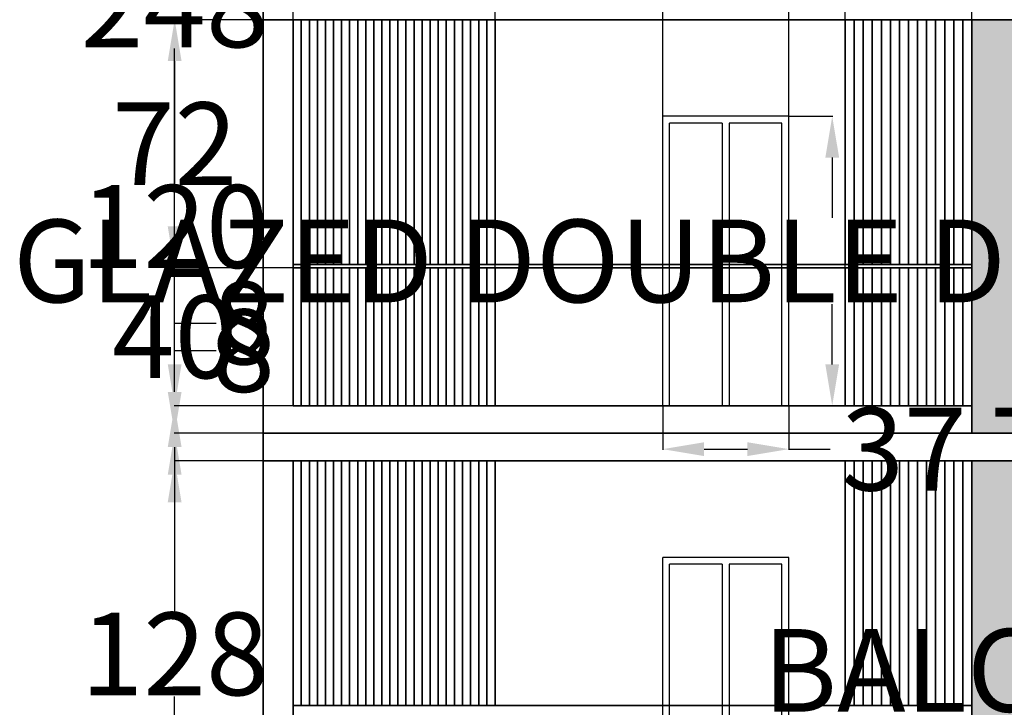
# Model space of a CAD drawing. Units: inches. Extents: x 172 to 828, y 190 to 777.
# Tile 2 of 9: x 188 to 474, y 408 to 607. Entities that reach past the tile are written whole.
import ezdxf

# ---------------------------------------------------------------- set-up
doc = ezdxf.new("R2010")
doc.units = ezdxf.units.IN
doc.header["$MEASUREMENT"] = 0
for name, color, linetype, lineweight in [('A-ANNO-DIMS', 2, 'Continuous', 18), ('A-DOOR', 4, 'Continuous', 25), ('A-ELEV', 7, 'Continuous', 35), ('A-ELEV-PATT', 8, 'Continuous', 13)]:
    doc.layers.add(name, color=color, linetype=linetype, lineweight=lineweight)
doc.styles.get("Standard").update_dxf_attribs({"font": 'arial.ttf'})
doc.dimstyles.get("Standard").update_dxf_attribs({"dimtxt": 24, "dimasz": 12, "dimexe": 0.18, "dimexo": 0.0625, "dimgap": 0.09, "dimtad": 0, "dimtih": 1, "dimtoh": 1, "dimdec": 0, "dimzin": 0, "dimdsep": 46, "dimlunit": 3, "dimtxsty": 'Standard', "dimcen": 0.09, "dimadec": 0, "dimazin": 0, "dimtfac": 1, "dimtdec": 0, "dimtofl": 0, "dimtmove": 0, "dimatfit": 3, "dimfxl": 1, "dimtolj": 1, "dimtzin": 0, "dimarcsym": 0})
pattern_1 = [(228.012788, (0.72, 1), (-8, -9), [0.134536, -13.319088]), (184.969741, (0.63, 0.9), (12, 1), [0.230868, -22.8559248]), (132.510447, (0.4, 0.88), (10, -11), [0.162788, -16.1160326]), (267.273689, (0.01, 0.63), (1, 20), [0.210238, -20.813558]), (292.833654, (0, 0.42), (-5, 12), [0.206155, -20.4093731]), (357.273689, (0.08, 0.23), (-20, 1), [0.210238, -20.813558]), (37.6942405, (0.29, 0.22), (-13, -10), [0.278029, -27.5248485]), (72.2553284, (0.51, 0.39), (7, 22), [0.262488, -25.9863215]), (121.4295656, (0.59, 0.64), (-8, 13), [0.21095, -20.8840731]), (175.236358, (0.48, 0.82), (11, -1), [0.240832, -11.8007626]), (222.397438, (0.24, 0.84), (-12, -11), [0.311448, -30.833375]), (138.814075, (1, 0.62), (-7, 6), [0.106301, -10.5238448]), (171.4692344, (0.92, 0.69), (13, -2), [0.202237, -20.0215114]), (225, (0.72, 0.72), (-1e-16, -1), [0.141421, -1.2727926]), (203.19859, (0.65, 0.84), (5, 2), [0.076158, -7.5396151]), (291.80141, (0.58, 0.81), (-1, 3), [0.107703, -5.2774618]), (30.963757, (0.62, 0.71), (3, 2), [0.174929, -5.6560229]), (161.56505, (0.77, 0.8), (2, -1), [0.126491, -3.0357867]), (16.38954, (0, 0.81), (10, 3), [0.1772, -17.5428451]), (70.346176, (0.17, 0.86), (-4, -11), [0.148661, -14.7174077]), (293.19859, (0.77, 1), (-2, 5), [0.152315, -7.4634581]), (343.61046, (0.83, 0.86), (-10, 3), [0.1772, -17.5428451]), (339.443955, (0, 0.19), (-5, 2), [0.17088, -8.3731237]), (294.775141, (0.16, 0.13), (-5, 11), [0.143178, -14.1746431]), (66.80141, (0.78, 0), (2, 5), [0.152315, -7.4634581]), (17.354025, (0.84, 0.14), (-13, -4), [0.167631, -16.5954236]), (69.443955, (0.29, 0), (-2, -5), [0.08544, -8.4585637]), (101.309932, (0.72, 0), (-1, 4), [0.05099, -5.0480295]), (165.963757, (0.71, 0.05), (3, -1), [0.206155, -3.9169506]), (186.009006, (0.51, 0.1), (10, 1), [0.19105, -18.9139232]), (303.690068, (0.62, 0.62), (-1, 2), [0.144222, -3.4613293]), (353.1572266, (0.7, 0.5), (17, -2), [0.251794, -24.9275626]), (60.945396, (0.95, 0.47), (-4, -7), [0.102956, -10.1926741]), (90, (1, 0.56), (-1, 1), [0.06, -0.94]), (120.256437, (0.49, 0.13), (4, -7), [0.138924, -13.75352]), (48.012788, (0.42, 0.25), (8, 9), [0.269072, -13.184552]), (0, (0.6, 0.45), (1, 1), [0.26, -0.74]), (325.3048465, (0.86, 0.45), (10, -7), [0.158114, -15.6532743]), (254.054604, (0.99, 0.36), (-1, -4), [0.145602, -7.1345079]), (207.6459754, (0.95, 0.22), (-19, -10), [0.237065, -23.4694742]), (175.426079, (0.74, 0.11), (-13, 1), [0.250799, -24.8290734])]

# ---------------------------------------------------------------- blocks, each defined once
blk = doc.blocks.new('DOOR-GLAZED-DBL')
for p, q in [((36.57, 84), (0, 84)), ((0, 0), (0, 84)), ((36.57, 0), (36.57, 84)), ((2, 0), (2, 82)), ((17.29, 82), (2, 82)), ((17.29, 82), (17.29, 0)), ((34.57, 82), (19.29, 82)), ((19.29, 82), (19.29, 0)), ((34.57, 0), (34.57, 82))]:
    blk.add_line(p, q)
blk = doc.blocks.new('*D4')
at = {"layer": 'A-ANNO-DIMS', "color": 0, "lineweight": -2, "transparency": 16777216}
for p, q in [((601.02, 471.8), (617.1, 471.8)), ((616.92, 459.8), (616.92, 431.1)), ((616.92, 377.39), (616.92, 406.09)), ((601.02, 365.39), (617.1, 365.39))]:
    blk.add_line(p, q, dxfattribs=at)
at = {"layer": 'A-ANNO-DIMS', "color": 0, "transparency": 16777216}
for points in [[(614.92, 459.8), (618.92, 459.8), (616.92, 471.8)], [(614.92, 377.39), (618.92, 377.39), (616.92, 365.39)]]:
    blk.add_solid(points, dxfattribs=at)
at = {"layer": 'Defpoints', "color": 0, "transparency": 16777216}
for p in [(600.96, 471.8), (616.92, 471.8), (600.96, 365.39)]:
    blk.add_point(p, dxfattribs=at)
at = {"layer": 'A-ANNO-DIMS', "color": 0, "transparency": 16777216, "insert": (616.92, 418.6), "char_height": 24, "attachment_point": 5}
blk.add_mtext('\\A1;BALCONY WINDOW 106 TYP.', dxfattribs=at)
blk = doc.blocks.new('*D6')
at = {"layer": 'A-ANNO-DIMS', "color": 0, "lineweight": -2, "transparency": 16777216}
for p, q in [((411.3, 579.39), (424.02, 579.39)), ((423.84, 567.39), (423.84, 549.9)), ((423.84, 507.39), (423.84, 524.88)), ((411.3, 495.39), (424.02, 495.39))]:
    blk.add_line(p, q, dxfattribs=at)
at = {"layer": 'A-ANNO-DIMS', "color": 0, "transparency": 16777216}
for points in [[(421.84, 567.39), (425.84, 567.39), (423.84, 579.39)], [(421.84, 507.39), (425.84, 507.39), (423.84, 495.39)]]:
    blk.add_solid(points, dxfattribs=at)
at = {"layer": 'Defpoints', "color": 0, "transparency": 16777216}
for p in [(411.24, 579.39), (423.84, 579.39), (411.24, 495.39)]:
    blk.add_point(p, dxfattribs=at)
at = {"layer": 'A-ANNO-DIMS', "color": 0, "transparency": 16777216, "insert": (423.84, 537.39), "char_height": 24, "attachment_point": 5}
blk.add_mtext('\\A1;GLAZED DOUBLE DOOR 84 TYP.', dxfattribs=at)
blk = doc.blocks.new('*D7')
at = {"layer": 'A-ANNO-DIMS', "color": 0, "lineweight": -2, "transparency": 16777216}
for p, q in [((374.66, 495.33), (374.66, 482.61)), ((411.24, 495.33), (411.24, 482.61)), ((386.66, 482.79), (399.24, 482.79)), ((411.24, 482.79), (423.24, 482.79))]:
    blk.add_line(p, q, dxfattribs=at)
at = {"layer": 'A-ANNO-DIMS', "color": 0, "transparency": 16777216}
for points in [[(386.66, 484.79), (386.66, 480.79), (374.66, 482.79)], [(399.24, 484.79), (399.24, 480.79), (411.24, 482.79)]]:
    blk.add_solid(points, dxfattribs=at)
at = {"layer": 'Defpoints', "color": 0, "transparency": 16777216}
for p in [(374.66, 495.39), (411.24, 495.39), (411.24, 482.79)]:
    blk.add_point(p, dxfattribs=at)
at = {"layer": 'A-ANNO-DIMS', "color": 0, "transparency": 16777216, "insert": (481.73, 482.79), "char_height": 24, "attachment_point": 5}
blk.add_mtext('\\A1;37 TYP.', dxfattribs=at)
blk = doc.blocks.new('*D10')
at = {"layer": 'A-ANNO-DIMS', "color": 0, "lineweight": -2, "transparency": 16777216}
for p, q in [((258.78, 231.45), (258.78, 761.27)), ((270.78, 761.09), (412.23, 761.09)), ((606.78, 761.09), (465.33, 761.09)), ((618.78, 735.45), (618.78, 761.27))]:
    blk.add_line(p, q, dxfattribs=at)
at = {"layer": 'A-ANNO-DIMS', "color": 0, "transparency": 16777216}
for points in [[(270.78, 763.09), (270.78, 759.09), (258.78, 761.09)], [(606.78, 763.09), (606.78, 759.09), (618.78, 761.09)]]:
    blk.add_solid(points, dxfattribs=at)
at = {"layer": 'Defpoints', "color": 0, "transparency": 16777216}
for p in [(618.78, 761.09), (618.78, 735.39), (258.78, 231.39)]:
    blk.add_point(p, dxfattribs=at)
at = {"layer": 'A-ANNO-DIMS', "color": 0, "transparency": 16777216, "insert": (438.78, 761.09), "char_height": 24, "attachment_point": 5}
blk.add_mtext('\\A1;360', dxfattribs=at)
blk = doc.blocks.new('*D13')
at = {"layer": 'A-ANNO-DIMS', "color": 0, "lineweight": -2, "transparency": 16777216}
for p, q in [((258.72, 487.39), (232.9, 487.39)), ((233.08, 475.39), (233.08, 435.74)), ((233.08, 371.39), (233.08, 411.05)), ((258.72, 359.39), (232.9, 359.39))]:
    blk.add_line(p, q, dxfattribs=at)
at = {"layer": 'A-ANNO-DIMS', "color": 0, "transparency": 16777216}
for points in [[(231.08, 475.39), (235.08, 475.39), (233.08, 487.39)], [(231.08, 371.39), (235.08, 371.39), (233.08, 359.39)]]:
    blk.add_solid(points, dxfattribs=at)
at = {"layer": 'Defpoints', "color": 0, "transparency": 16777216}
for p in [(233.08, 487.39), (258.78, 487.39), (258.78, 359.39)]:
    blk.add_point(p, dxfattribs=at)
at = {"layer": 'A-ANNO-DIMS', "color": 0, "transparency": 16777216, "insert": (233.08, 423.39), "char_height": 24, "attachment_point": 5}
blk.add_mtext('\\A1;128', dxfattribs=at)
blk = doc.blocks.new('*D14')
at = {"layer": 'A-ANNO-DIMS', "color": 0, "lineweight": -2, "transparency": 16777216}
for p, q in [((258.72, 735.39), (232.9, 735.39)), ((233.08, 723.39), (233.08, 623.74)), ((233.08, 499.39), (233.08, 599.05)), ((258.72, 487.39), (232.9, 487.39))]:
    blk.add_line(p, q, dxfattribs=at)
at = {"layer": 'A-ANNO-DIMS', "color": 0, "transparency": 16777216}
for points in [[(231.08, 723.39), (235.08, 723.39), (233.08, 735.39)], [(231.08, 499.39), (235.08, 499.39), (233.08, 487.39)]]:
    blk.add_solid(points, dxfattribs=at)
at = {"layer": 'Defpoints', "color": 0, "transparency": 16777216}
for p in [(233.08, 735.39), (258.78, 735.39), (258.78, 487.39)]:
    blk.add_point(p, dxfattribs=at)
at = {"layer": 'A-ANNO-DIMS', "color": 0, "transparency": 16777216, "insert": (233.08, 611.39), "char_height": 24, "attachment_point": 5}
blk.add_mtext('\\A1;248', dxfattribs=at)
blk = doc.blocks.new('*D67')
at = {"layer": 'A-ANNO-DIMS', "color": 0, "lineweight": -2, "transparency": 16777216}
for p, q in [((233.08, 499.39), (233.08, 511.39)), ((233.08, 511.39), (245.08, 511.39)), ((258.72, 487.39), (232.9, 487.39)), ((258.72, 479.39), (232.9, 479.39)), ((233.08, 467.39), (233.08, 455.39))]:
    blk.add_line(p, q, dxfattribs=at)
at = {"layer": 'A-ANNO-DIMS', "color": 0, "transparency": 16777216}
for points in [[(231.08, 499.39), (235.08, 499.39), (233.08, 487.39)], [(231.08, 467.39), (235.08, 467.39), (233.08, 479.39)]]:
    blk.add_solid(points, dxfattribs=at)
at = {"layer": 'Defpoints', "color": 0, "transparency": 16777216}
for p in [(233.08, 487.39), (258.78, 487.39), (258.78, 479.39)]:
    blk.add_point(p, dxfattribs=at)
at = {"layer": 'A-ANNO-DIMS', "color": 0, "transparency": 16777216, "insert": (253.08, 511.39), "char_height": 24, "attachment_point": 5}
blk.add_mtext('\\A1;8', dxfattribs=at)
blk = doc.blocks.new('*D68')
at = {"layer": 'A-ANNO-DIMS', "color": 0, "lineweight": -2, "transparency": 16777216}
for p, q in [((258.72, 607.39), (232.9, 607.39)), ((233.08, 595.39), (233.08, 559.74)), ((233.08, 499.39), (233.08, 535.05)), ((258.72, 487.39), (232.9, 487.39))]:
    blk.add_line(p, q, dxfattribs=at)
at = {"layer": 'A-ANNO-DIMS', "color": 0, "transparency": 16777216}
for points in [[(231.08, 595.39), (235.08, 595.39), (233.08, 607.39)], [(231.08, 499.39), (235.08, 499.39), (233.08, 487.39)]]:
    blk.add_solid(points, dxfattribs=at)
at = {"layer": 'Defpoints', "color": 0, "transparency": 16777216}
for p in [(233.08, 607.39), (258.78, 607.39), (258.78, 487.39)]:
    blk.add_point(p, dxfattribs=at)
at = {"layer": 'A-ANNO-DIMS', "color": 0, "transparency": 16777216, "insert": (233.08, 547.39), "char_height": 24, "attachment_point": 5}
blk.add_mtext('\\A1;120', dxfattribs=at)
blk = doc.blocks.new('*D69')
at = {"layer": 'A-ANNO-DIMS', "color": 0, "lineweight": -2, "transparency": 16777216}
for p, q in [((233.08, 627.39), (233.08, 639.39)), ((233.08, 639.39), (245.08, 639.39)), ((267.42, 615.39), (232.9, 615.39)), ((258.72, 607.39), (232.9, 607.39)), ((233.08, 595.39), (233.08, 583.39))]:
    blk.add_line(p, q, dxfattribs=at)
at = {"layer": 'A-ANNO-DIMS', "color": 0, "transparency": 16777216}
for points in [[(231.08, 627.39), (235.08, 627.39), (233.08, 615.39)], [(231.08, 595.39), (235.08, 595.39), (233.08, 607.39)]]:
    blk.add_solid(points, dxfattribs=at)
at = {"layer": 'Defpoints', "color": 0, "transparency": 16777216}
for p in [(233.08, 615.39), (267.48, 615.39), (258.78, 607.39)]:
    blk.add_point(p, dxfattribs=at)
at = {"layer": 'A-ANNO-DIMS', "color": 0, "transparency": 16777216, "insert": (253.08, 639.39), "char_height": 24, "attachment_point": 5}
blk.add_mtext('\\A1;8', dxfattribs=at)
blk = doc.blocks.new('*D70')
at = {"layer": 'A-ANNO-DIMS', "color": 0, "lineweight": -2, "transparency": 16777216}
for p, q in [((233.08, 507.39), (233.08, 519.39)), ((233.08, 519.39), (245.08, 519.39)), ((267.42, 495.39), (232.9, 495.39)), ((258.72, 487.39), (232.9, 487.39)), ((233.08, 475.39), (233.08, 463.39))]:
    blk.add_line(p, q, dxfattribs=at)
at = {"layer": 'A-ANNO-DIMS', "color": 0, "transparency": 16777216}
for points in [[(231.08, 507.39), (235.08, 507.39), (233.08, 495.39)], [(231.08, 475.39), (235.08, 475.39), (233.08, 487.39)]]:
    blk.add_solid(points, dxfattribs=at)
at = {"layer": 'Defpoints', "color": 0, "transparency": 16777216}
for p in [(233.08, 495.39), (267.48, 495.39), (258.78, 487.39)]:
    blk.add_point(p, dxfattribs=at)
at = {"layer": 'A-ANNO-DIMS', "color": 0, "transparency": 16777216, "insert": (253.08, 519.39), "char_height": 24, "attachment_point": 5}
blk.add_mtext('\\A1;8', dxfattribs=at)
blk = doc.blocks.new('*D71')
at = {"layer": 'A-ANNO-DIMS', "color": 0, "lineweight": -2, "transparency": 16777216}
for p, q in [((233.079175, 547.392291), (233.079175, 559.392291)), ((267.419715, 535.392291), (232.899175, 535.392291)), ((267.419715, 495.392291), (232.899175, 495.392291)), ((233.079175, 483.392291), (233.079175, 471.392291))]:
    blk.add_line(p, q, dxfattribs=at)
at = {"layer": 'A-ANNO-DIMS', "color": 0, "transparency": 16777216}
for points in [[(231.079175, 547.392291), (235.079175, 547.392291), (233.079175, 535.392291)], [(231.079175, 483.392291), (235.079175, 483.392291), (233.079175, 495.392291)]]:
    blk.add_solid(points, dxfattribs=at)
at = {"layer": 'Defpoints', "color": 0, "transparency": 16777216}
for p in [(233.079175, 535.392291), (267.482215, 535.392291), (267.482215, 495.392291)]:
    blk.add_point(p, dxfattribs=at)
at = {"layer": 'A-ANNO-DIMS', "color": 0, "transparency": 16777216, "insert": (233.079175, 515.392291), "char_height": 24, "attachment_point": 5}
blk.add_mtext('\\A1;40', dxfattribs=at)
blk = doc.blocks.new('*D72')
at = {"layer": 'A-ANNO-DIMS', "color": 0, "lineweight": -2, "transparency": 16777216}
for p, q in [((267.42, 607.39), (232.9, 607.39)), ((233.08, 595.39), (233.08, 583.53)), ((233.08, 547.39), (233.08, 559.25)), ((267.42, 535.39), (232.9, 535.39))]:
    blk.add_line(p, q, dxfattribs=at)
at = {"layer": 'A-ANNO-DIMS', "color": 0, "transparency": 16777216}
for points in [[(231.08, 595.39), (235.08, 595.39), (233.08, 607.39)], [(231.08, 547.39), (235.08, 547.39), (233.08, 535.39)]]:
    blk.add_solid(points, dxfattribs=at)
at = {"layer": 'Defpoints', "color": 0, "transparency": 16777216}
for p in [(233.08, 607.39), (267.48, 607.39), (267.48, 535.39)]:
    blk.add_point(p, dxfattribs=at)
at = {"layer": 'A-ANNO-DIMS', "color": 0, "transparency": 16777216, "insert": (233.08, 571.39), "char_height": 24, "attachment_point": 5}
blk.add_mtext('\\A1;72', dxfattribs=at)
blk = doc.blocks.new('*D73')
at = {"layer": 'A-ANNO-DIMS', "color": 0, "lineweight": -2, "transparency": 16777216}
for p, q in [((246.78, 761.09), (234.78, 761.09)), ((258.78, 607.45), (258.78, 761.27)), ((267.48, 495.45), (267.48, 761.27)), ((279.48, 761.09), (291.48, 761.09))]:
    blk.add_line(p, q, dxfattribs=at)
at = {"layer": 'A-ANNO-DIMS', "color": 0, "transparency": 16777216}
for points in [[(246.78, 763.09), (246.78, 759.09), (258.78, 761.09)], [(279.48, 763.09), (279.48, 759.09), (267.48, 761.09)]]:
    blk.add_solid(points, dxfattribs=at)
at = {"layer": 'Defpoints', "color": 0, "transparency": 16777216}
for p in [(267.48, 761.09), (258.78, 607.39), (267.48, 495.39)]:
    blk.add_point(p, dxfattribs=at)
at = {"layer": 'A-ANNO-DIMS', "color": 0, "transparency": 16777216, "insert": (332.08, 761.09), "char_height": 24, "attachment_point": 5}
blk.add_mtext('\\A1;8.703', dxfattribs=at)
blk = doc.blocks.new('*D74')
at = {"layer": 'A-ANNO-DIMS', "color": 0, "lineweight": -2, "transparency": 16777216}
for p, q in [((267.48, 495.45), (267.48, 761.27)), ((279.48, 761.09), (314.08, 761.09)), ((326.08, 495.45), (326.08, 761.27)), ((326.08, 761.09), (338.08, 761.09))]:
    blk.add_line(p, q, dxfattribs=at)
at = {"layer": 'A-ANNO-DIMS', "color": 0, "transparency": 16777216}
for points in [[(279.48, 763.09), (279.48, 759.09), (267.48, 761.09)], [(314.08, 763.09), (314.08, 759.09), (326.08, 761.09)]]:
    blk.add_solid(points, dxfattribs=at)
at = {"layer": 'Defpoints', "color": 0, "transparency": 16777216}
for p in [(326.08, 761.09), (267.48, 495.39), (326.08, 495.39)]:
    blk.add_point(p, dxfattribs=at)
at = {"layer": 'A-ANNO-DIMS', "color": 0, "transparency": 16777216, "insert": (378.68, 761.09), "char_height": 24, "attachment_point": 5}
blk.add_mtext('\\A1;58.59', dxfattribs=at)
blk = doc.blocks.new('*D75')
at = {"layer": 'A-ANNO-DIMS', "color": 0, "lineweight": -2, "transparency": 16777216}
for p, q in [((326.08, 495.45), (326.08, 761.27)), ((338.08, 761.09), (362.66, 761.09)), ((374.66, 495.45), (374.66, 761.27)), ((374.66, 761.09), (386.66, 761.09))]:
    blk.add_line(p, q, dxfattribs=at)
at = {"layer": 'A-ANNO-DIMS', "color": 0, "transparency": 16777216}
for points in [[(338.08, 763.09), (338.08, 759.09), (326.08, 761.09)], [(362.66, 763.09), (362.66, 759.09), (374.66, 761.09)]]:
    blk.add_solid(points, dxfattribs=at)
at = {"layer": 'Defpoints', "color": 0, "transparency": 16777216}
for p in [(374.66, 761.09), (326.08, 495.39), (374.66, 495.39)]:
    blk.add_point(p, dxfattribs=at)
at = {"layer": 'A-ANNO-DIMS', "color": 0, "transparency": 16777216, "insert": (427.75, 761.09), "char_height": 24, "attachment_point": 5}
blk.add_mtext('\\A1;48.59', dxfattribs=at)
blk = doc.blocks.new('*D76')
at = {"layer": 'A-ANNO-DIMS', "color": 0, "lineweight": -2, "transparency": 16777216}
for p, q in [((399.24, 761.09), (387.24, 761.09)), ((411.24, 495.45), (411.24, 761.27)), ((427.59, 495.45), (427.59, 761.27)), ((439.59, 761.09), (451.59, 761.09))]:
    blk.add_line(p, q, dxfattribs=at)
at = {"layer": 'A-ANNO-DIMS', "color": 0, "transparency": 16777216}
for points in [[(399.24, 763.09), (399.24, 759.09), (411.24, 761.09)], [(439.59, 763.09), (439.59, 759.09), (427.59, 761.09)]]:
    blk.add_solid(points, dxfattribs=at)
at = {"layer": 'Defpoints', "color": 0, "transparency": 16777216}
for p in [(427.59, 761.09), (411.24, 495.39), (427.59, 495.39)]:
    blk.add_point(p, dxfattribs=at)
at = {"layer": 'A-ANNO-DIMS', "color": 0, "transparency": 16777216, "insert": (500.36, 761.09), "char_height": 24, "attachment_point": 5}
blk.add_mtext('\\A1;16.356', dxfattribs=at)
blk = doc.blocks.new('*D77')
at = {"layer": 'A-ANNO-DIMS', "color": 0, "lineweight": -2, "transparency": 16777216}
for p, q in [((427.59, 495.45), (427.59, 761.27)), ((439.59, 761.09), (452.34, 761.09)), ((464.34, 495.45), (464.34, 761.27)), ((464.34, 761.09), (476.34, 761.09))]:
    blk.add_line(p, q, dxfattribs=at)
at = {"layer": 'A-ANNO-DIMS', "color": 0, "transparency": 16777216}
for points in [[(439.59, 763.09), (439.59, 759.09), (427.59, 761.09)], [(452.34, 763.09), (452.34, 759.09), (464.34, 761.09)]]:
    blk.add_solid(points, dxfattribs=at)
at = {"layer": 'Defpoints', "color": 0, "transparency": 16777216}
for p in [(464.34, 761.09), (427.59, 495.39), (464.34, 495.39)]:
    blk.add_point(p, dxfattribs=at)
at = {"layer": 'A-ANNO-DIMS', "color": 0, "transparency": 16777216, "insert": (516.86, 761.09), "char_height": 24, "attachment_point": 5}
blk.add_mtext('\\A1;36.74', dxfattribs=at)

msp = doc.modelspace()

# ---------------------------------------------------------------- hatches: boundary and pattern name
at = {"layer": 'A-ELEV-PATT'}
h = msp.add_hatch(dxfattribs=at)
h.set_pattern_fill('GRAVEL', color=256)
h.set_pattern_definition(pattern_1)
h.paths.add_polyline_path([(438.7792, 351.3923), (414.7792, 351.3923), (414.7792, 249.3923), (438.7792, 249.3923)])
h.paths.add_polyline_path([(480.7792, 351.3923), (456.7792, 351.3923), (456.7792, 249.3923), (480.7792, 249.3923)])
h.paths.add_polyline_path([(488.4232, 479.3923), (472.3356, 479.3923), (472.3356, 359.3923), (488.4232, 359.3923)])
h.paths.add_polyline_path([(488.4232, 607.3923), (472.3356, 607.3923), (472.3356, 487.3923), (488.4232, 487.3923)])
h = msp.add_hatch(dxfattribs=at)
h.set_pattern_fill('GRAVEL', color=256)
h.set_pattern_definition(pattern_1)
h.paths.add_polyline_path([(480.7792, 351.3923), (456.7792, 351.3923), (456.7792, 249.3923), (480.7792, 249.3923)])
h.paths.add_polyline_path([(488.4232, 479.3923), (472.3356, 479.3923), (472.3356, 359.3923), (488.4232, 359.3923)])
h.paths.add_polyline_path([(488.4232, 607.3923), (472.3356, 607.3923), (472.3356, 487.3923), (488.4232, 487.3923)])
h = msp.add_hatch(dxfattribs=at)
h.set_pattern_fill('GRAVEL', color=256, scale=20)
h.set_pattern_definition([(228.01279, (14.4, 20), (-160, -180), [2.69072, -266.38176]), (184.96974, (12.6, 18), (240, 20), [4.61736, -457.1185]), (132.51045, (8, 17.6), (200, -220), [3.25576, -322.32065]), (267.27369, (0.2, 12.6), (20, 400), [4.20476, -416.27116]), (292.83365, (0, 8.4), (-100, 240), [4.1231, -408.18746]), (357.27369, (1.6, 4.6), (-400, 20), [4.20476, -416.27116]), (37.69424, (5.8, 4.4), (-260, -200), [5.56058, -550.49697]), (72.25533, (10.2, 7.8), (140, 440), [5.24976, -519.72643]), (121.42957, (11.8, 12.8), (-160, 260), [4.219, -417.68146]), (175.23636, (9.6, 16.4), (220, -20), [4.81664, -236.01525]), (222.39744, (4.8, 16.8), (-240, -220), [6.22896, -616.6675]), (138.81407, (20, 12.4), (-140, 120), [2.126, -210.4769]), (171.46923, (18.4, 13.8), (260, -40), [4.04474, -400.43023]), (225, (14.4, 14.4), (-2e-15, -20), [2.8284, -25.45585]), (203.1986, (13, 16.8), (100, 40), [1.52316, -150.7923]), (291.8014, (11.6, 16.2), (-20, 60), [2.15406, -105.54924]), (30.96376, (12.4, 14.2), (60, 40), [3.4986, -113.12046]), (161.56505, (15.4, 16), (40, -20), [2.5298, -60.71573]), (16.38954, (0, 16.2), (200, 60), [3.544, -350.8569]), (70.34618, (3.4, 17.2), (-80, -220), [2.97322, -294.34815]), (293.1986, (15.4, 20), (-40, 100), [3.0463, -149.26916]), (343.61046, (16.6, 17.2), (-200, 60), [3.544, -350.8569]), (339.44395, (0, 3.8), (-100, 40), [3.4176, -167.46247]), (294.77514, (3.2, 2.6), (-100, 220), [2.86356, -283.49286]), (66.8014, (15.6, 0), (40, 100), [3.0463, -149.26916]), (17.35402, (16.8, 2.8), (-260, -80), [3.35262, -331.90847]), (69.44395, (5.8, 0), (-40, -100), [1.7088, -169.17127]), (101.30993, (14.4, 0), (-20, 80), [1.0198, -100.9606]), (165.96376, (14.2, 1), (60, -20), [4.1231, -78.339]), (186.009, (10.2, 2), (200, 20), [3.821, -378.27846]), (303.6901, (12.4, 12.4), (-20, 40), [2.88444, -69.2266]), (353.15723, (14, 10), (340, -40), [5.03588, -498.55125]), (60.9454, (19, 9.4), (-80, -140), [2.0591, -203.8535]), (90, (20, 11.2), (-20, 20), [1.2, -18.8]), (120.25644, (9.8, 2.6), (80, -140), [2.77848, -275.0704]), (48.01279, (8.4, 5), (160, 180), [5.38144, -263.69104]), (0, (12, 9), (20, 20), [5.2, -14.8]), (325.30485, (17.2, 9), (200, -140), [3.16228, -313.0655]), (254.0546, (19.8, 7.2), (-20, -80), [2.91204, -142.69016]), (207.64598, (19, 4.4), (-380, -200), [4.7413, -469.38948]), (175.42608, (14.8, 2.2), (-260, 20), [5.01598, -496.58147])])
h.paths.add_polyline_path([(480.7792, 351.3923), (456.7792, 351.3923), (456.7792, 249.3923), (480.7792, 249.3923)])
h.paths.add_polyline_path([(472.3356, 479.3923), (464.3356, 479.3923), (464.3356, 359.3923), (472.3356, 359.3923)])
h.paths.add_polyline_path([(488.4232, 479.3923), (472.3356, 479.3923), (472.3356, 359.3923), (488.4232, 359.3923)])
h.paths.add_polyline_path([(472.3356, 607.3923), (464.3356, 607.3923), (464.3356, 487.3923), (472.3356, 487.3923)])
h.paths.add_polyline_path([(488.4232, 607.3923), (472.3356, 607.3923), (472.3356, 487.3923), (488.4232, 487.3923)])

# ---------------------------------------------------------------- linework, layer by layer
at = {"layer": 'A-ELEV'}
for p, q in [((258.7792, 487.3923), (258.7792, 735.3923)), ((606.8158, 607.3923), (258.7792, 607.3923)), ((606.8158, 607.3923), (258.7792, 607.3923)), ((267.4822, 495.3923), (267.4822, 607.3923)), ((269.8186, 536.3923), (269.8186, 607.3923)), ((272.155, 536.3923), (272.155, 607.3923)), ((274.4914, 536.3923), (274.4914, 607.3923)), ((276.8278, 536.3923), (276.8278, 607.3923)), ((279.1642, 536.3923), (279.1642, 607.3923)), ((281.5006, 536.3923), (281.5006, 607.3923)), ((283.837, 536.3923), (283.837, 607.3923)), ((286.1735, 536.3923), (286.1735, 607.3923)), ((288.5099, 536.3923), (288.5099, 607.3923)), ((290.8463, 536.3923), (290.8463, 607.3923)), ((293.1827, 536.3923), (293.1827, 607.3923)), ((295.5191, 536.3923), (295.5191, 607.3923)), ((297.8555, 536.3923), (297.8555, 607.3923)), ((300.1919, 536.3923), (300.1919, 607.3923)), ((302.5283, 536.3923), (302.5283, 607.3923)), ((304.8647, 536.3923), (304.8647, 607.3923)), ((307.2011, 536.3923), (307.2011, 607.3923)), ((309.5375, 536.3923), (309.5375, 607.3923)), ((311.8739, 536.3923), (311.8739, 607.3923)), ((314.2715, 536.3923), (314.2715, 607.3923)), ((316.6079, 536.3923), (316.6079, 607.3923)), ((318.9443, 536.3923), (318.9443, 607.3923)), ((321.3419, 536.3923), (321.3419, 607.3923)), ((323.6783, 536.3923), (323.6783, 607.3923)), ((326.0147, 536.3923), (326.0147, 607.3923)), ((427.5926, 607.3923), (427.5926, 536.3923)), ((427.5926, 536.3923), (427.5926, 607.3923)), ((430.2171, 607.3923), (430.2171, 536.3923)), ((432.8416, 607.3923), (432.8416, 536.3923)), ((435.4661, 607.3923), (435.4661, 536.3923)), ((438.0906, 607.3923), (438.0906, 536.3923)), ((440.7151, 607.3923), (440.7151, 536.3923)), ((443.3396, 607.3923), (443.3396, 536.3923)), ((445.9641, 607.3923), (445.9641, 536.3923)), ((448.5886, 607.3923), (448.5886, 536.3923)), ((451.2131, 607.3923), (451.2131, 536.3923)), ((453.8376, 607.3923), (453.8376, 536.3923)), ((456.4621, 607.3923), (456.4621, 536.3923)), ((459.0866, 607.3923), (459.0866, 536.3923)), ((461.7111, 607.3923), (461.7111, 536.3923)), ((464.3356, 607.3923), (464.3356, 487.3923)), ((464.3356, 536.3923), (267.4822, 536.3923)), ((464.3356, 535.3923), (267.4822, 535.3923)), ((269.8186, 495.3923), (269.8186, 535.3923)), ((272.155, 495.3923), (272.155, 535.3923)), ((274.4914, 495.3923), (274.4914, 535.3923)), ((276.8278, 495.3923), (276.8278, 535.3923)), ((279.1642, 495.3923), (279.1642, 535.3923)), ((281.5006, 495.3923), (281.5006, 535.3923)), ((283.837, 495.3923), (283.837, 535.3923)), ((286.1735, 495.3923), (286.1735, 535.3923)), ((288.5099, 495.3923), (288.5099, 535.3923)), ((290.8463, 495.3923), (290.8463, 535.3923)), ((293.1827, 495.3923), (293.1827, 535.3923)), ((295.5191, 495.3923), (295.5191, 535.3923)), ((297.8555, 495.3923), (297.8555, 535.3923)), ((300.1919, 495.3923), (300.1919, 535.3923)), ((302.5283, 495.3923), (302.5283, 535.3923)), ((304.8647, 495.3923), (304.8647, 535.3923)), ((307.2011, 495.3923), (307.2011, 535.3923)), ((309.5375, 495.3923), (309.5375, 535.3923)), ((311.8739, 495.3923), (311.8739, 535.3923)), ((314.2715, 495.3923), (314.2715, 535.3923)), ((316.6079, 495.3923), (316.6079, 535.3923)), ((318.9443, 495.3923), (318.9443, 535.3923)), ((321.3419, 495.3923), (321.3419, 535.3923)), ((323.6783, 495.3923), (323.6783, 535.3923)), ((326.0759, 495.3923), (326.0759, 535.3923)), ((427.5926, 495.3923), (427.5926, 535.3923)), ((427.5926, 535.3923), (427.5926, 495.3923)), ((430.2171, 535.3923), (430.2171, 495.3923)), ((432.8416, 535.3923), (432.8416, 495.3923)), ((435.4661, 535.3923), (435.4661, 495.3923)), ((438.0906, 535.3923), (438.0906, 495.3923)), ((440.7151, 535.3923), (440.7151, 495.3923)), ((443.3396, 535.3923), (443.3396, 495.3923)), ((445.9641, 535.3923), (445.9641, 495.3923)), ((448.5886, 535.3923), (448.5886, 495.3923)), ((451.2131, 535.3923), (451.2131, 495.3923)), ((453.8376, 535.3923), (453.8376, 495.3923)), ((456.4621, 535.3923), (456.4621, 495.3923)), ((459.0866, 535.3923), (459.0866, 495.3923)), ((461.7111, 535.3923), (461.7111, 495.3923)), ((464.3356, 495.3923), (267.4822, 495.3923)), ((606.8158, 487.3923), (258.7792, 487.3923)), ((258.7792, 487.3923), (258.7792, 359.3923)), ((472.3356, 487.3923), (393.1206, 487.3923)), ((606.8158, 479.3923), (258.7792, 479.3923)), ((258.7792, 359.3923), (258.7792, 479.3923)), ((267.4822, 367.3923), (267.4822, 479.3923)), ((269.8186, 408.3923), (269.8186, 479.3923)), ((272.155, 408.3923), (272.155, 479.3923)), ((274.4914, 408.3923), (274.4914, 479.3923)), ((276.8278, 408.3923), (276.8278, 479.3923)), ((279.1642, 408.3923), (279.1642, 479.3923)), ((281.5006, 408.3923), (281.5006, 479.3923)), ((283.837, 408.3923), (283.837, 479.3923)), ((286.1735, 408.3923), (286.1735, 479.3923)), ((288.5099, 408.3923), (288.5099, 479.3923)), ((290.8463, 408.3923), (290.8463, 479.3923)), ((293.1827, 408.3923), (293.1827, 479.3923)), ((295.5191, 408.3923), (295.5191, 479.3923)), ((297.8555, 408.3923), (297.8555, 479.3923)), ((300.1919, 408.3923), (300.1919, 479.3923)), ((302.5283, 408.3923), (302.5283, 479.3923)), ((304.8647, 408.3923), (304.8647, 479.3923)), ((307.2011, 408.3923), (307.2011, 479.3923)), ((309.5375, 408.3923), (309.5375, 479.3923)), ((311.8739, 408.3923), (311.8739, 479.3923)), ((314.2715, 408.3923), (314.2715, 479.3923)), ((316.6079, 408.3923), (316.6079, 479.3923)), ((318.9443, 408.3923), (318.9443, 479.3923)), ((321.3419, 408.3923), (321.3419, 479.3923)), ((323.6783, 408.3923), (323.6783, 479.3923)), ((326.0147, 408.3923), (326.0147, 479.3923)), ((427.5926, 479.3923), (427.5926, 408.3923)), ((427.5926, 408.3923), (427.5926, 479.3923)), ((430.2171, 479.3923), (430.2171, 408.3923)), ((432.8416, 479.3923), (432.8416, 408.3923)), ((435.4661, 479.3923), (435.4661, 408.3923)), ((438.0906, 479.3923), (438.0906, 408.3923)), ((440.7151, 479.3923), (440.7151, 408.3923)), ((443.3396, 479.3923), (443.3396, 408.3923)), ((445.9641, 479.3923), (445.9641, 408.3923)), ((448.5886, 479.3923), (448.5886, 408.3923)), ((451.2131, 479.3923), (451.2131, 408.3923)), ((453.8376, 479.3923), (453.8376, 408.3923)), ((456.4621, 479.3923), (456.4621, 408.3923)), ((459.0866, 479.3923), (459.0866, 408.3923)), ((461.7111, 479.3923), (461.7111, 408.3923)), ((464.3356, 479.3923), (464.3356, 359.3923)), ((464.3356, 408.3923), (267.4822, 408.3923))]:
    msp.add_line(p, q, dxfattribs=at)

# ---------------------------------------------------------------- block references
at = {"layer": 'A-DOOR'}
for p in [(374.663, 495.392), (374.663, 367.392)]:
    msp.add_blockref('DOOR-GLAZED-DBL', p, dxfattribs=at)

# ---------------------------------------------------------------- dimensions: what is measured, and where the dimension line sits
at = {"layer": 'A-ANNO-DIMS'}
for base, p1, p2, override, picture, middle in [((267.4822, 761.0923), (258.7792, 607.3923), (267.4822, 495.3923), {"dimdec": 3, "dimlfac": 1, "dimrnd": 0, "dimzin": 0, "dimdsep": 46, "dimlunit": 2}, '*D73', (332.0824, 761.0923)), ((618.7792, 761.0923), (258.7792, 231.3923), (618.7792, 735.3923), {"dimdec": 0, "dimlfac": 1, "dimrnd": 0, "dimzin": 0, "dimdsep": 46, "dimlunit": 2}, '*D10', (438.7792, 761.0923)), ((326.0759, 761.0923), (267.4822, 495.3923), (326.0759, 495.3923), {"dimdec": 2, "dimlfac": 1, "dimrnd": 0, "dimzin": 0, "dimdsep": 46, "dimlunit": 2}, '*D74', (378.6843, 761.0923)), ((374.6632, 761.0923), (326.0759, 495.3923), (374.6632, 495.3923), {"dimdec": 2, "dimlfac": 1, "dimrnd": 0, "dimzin": 0, "dimdsep": 46, "dimlunit": 2}, '*D75', (427.7546, 761.0923)), ((427.5926, 761.0923), (411.2362, 495.3923), (427.5926, 495.3923), {"dimdec": 3, "dimlfac": 1, "dimrnd": 0, "dimzin": 0, "dimdsep": 46, "dimlunit": 2}, '*D76', (500.362, 761.0923)), ((464.3356, 761.0923), (427.5926, 495.3923), (464.3356, 495.3923), {"dimdec": 2, "dimlfac": 1, "dimrnd": 0, "dimzin": 0, "dimdsep": 46, "dimlunit": 2}, '*D77', (516.8622, 761.0923))]:
    dim = msp.add_linear_dim(base=base, p1=p1, p2=p2, dimstyle='Standard', override=override, dxfattribs=at)
    dim.commit()
    dim.dimension.update_dxf_attribs({"geometry": picture, "text_midpoint": middle})
for base, p1, p2, picture, middle in [((233.0792, 735.3923), (258.7792, 487.3923), (258.7792, 735.3923), '*D14', (233.0792, 611.3923)), ((233.0792, 615.3923), (258.7792, 607.3923), (267.4822, 615.3923), '*D69', (253.0764, 639.3923)), ((233.0792, 607.3923), (258.7792, 487.3923), (258.7792, 607.3923), '*D68', (233.0792, 547.3923)), ((233.0792, 607.3923), (267.4822, 535.3923), (267.4822, 607.3923), '*D72', (233.0792, 571.3923)), ((233.0792, 535.3923), (267.4822, 495.3923), (267.4822, 535.3923), '*D71', (233.0792, 515.3923)), ((233.0792, 495.3923), (258.7792, 487.3923), (267.4822, 495.3923), '*D70', (253.0764, 519.3923)), ((233.0792, 487.3923), (258.7792, 479.3923), (258.7792, 487.3923), '*D67', (253.0764, 511.3923)), ((233.0792, 487.3923), (258.7792, 359.3923), (258.7792, 487.3923), '*D13', (233.0792, 423.3923))]:
    dim = msp.add_linear_dim(base=base, p1=p1, p2=p2, angle=90, dimstyle='Standard', override={"dimdec": 0, "dimlfac": 1, "dimrnd": 0, "dimzin": 0, "dimdsep": 46, "dimlunit": 2}, dxfattribs=at)
    dim.commit()
    dim.dimension.update_dxf_attribs({"geometry": picture, "text_midpoint": middle})
for base, p1, p2, text, picture, middle in [((423.8362, 579.3923), (411.2362, 495.3923), (411.2362, 579.3923), 'GLAZED DOUBLE DOOR <> TYP.', '*D6', (423.8362, 537.3923)), ((616.9208, 471.8013), (600.9594, 365.3923), (600.9594, 471.8013), 'BALCONY WINDOW <> TYP.', '*D4', (616.9208, 418.5968))]:
    dim = msp.add_linear_dim(base=base, p1=p1, p2=p2, angle=90, text=text, dimstyle='Standard', override={"dimdec": 0, "dimlfac": 1, "dimrnd": 0, "dimzin": 0, "dimdsep": 46, "dimlunit": 2}, dxfattribs=at)
    dim.commit()
    dim.dimension.update_dxf_attribs({"geometry": picture, "text_midpoint": middle})
dim = msp.add_linear_dim(base=(411.2362, 482.7923), p1=(374.6632, 495.3923), p2=(411.2362, 495.3923), text='<> TYP.', dimstyle='Standard', override={"dimdec": 0, "dimlfac": 1, "dimrnd": 0, "dimzin": 0, "dimdsep": 46, "dimlunit": 2}, dxfattribs=at)
dim.commit()
dim.dimension.update_dxf_attribs({"geometry": '*D7', "text_midpoint": (481.7301, 482.7923)})

doc.saveas('drawing.dxf')
